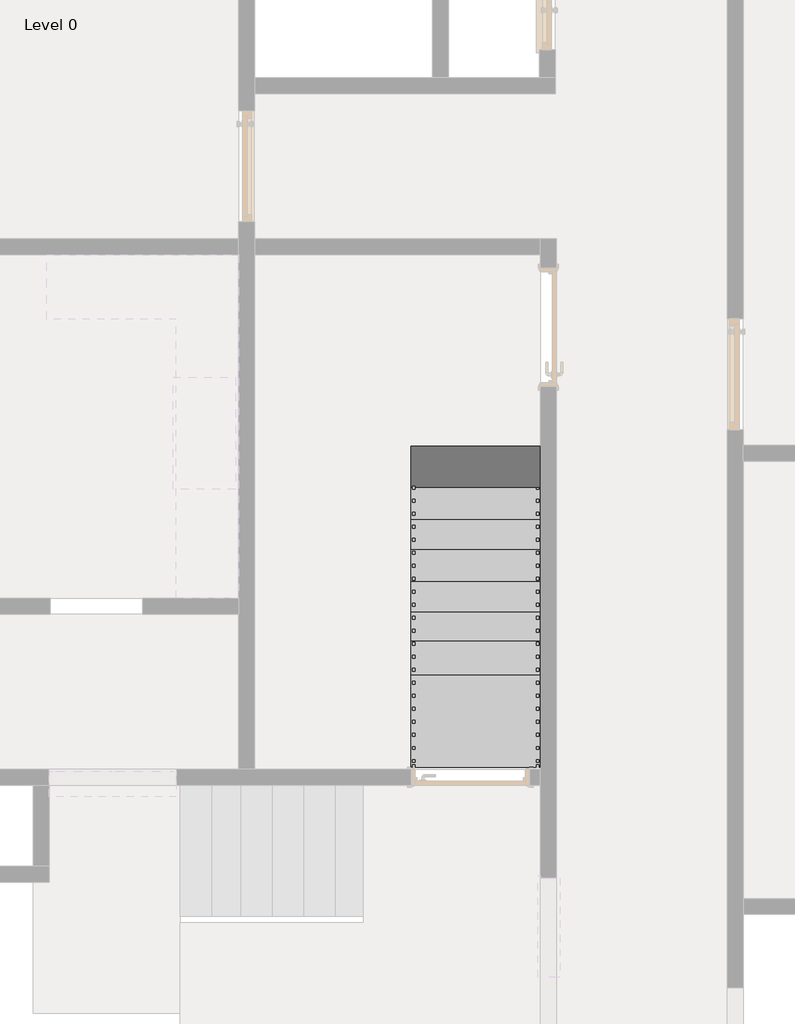
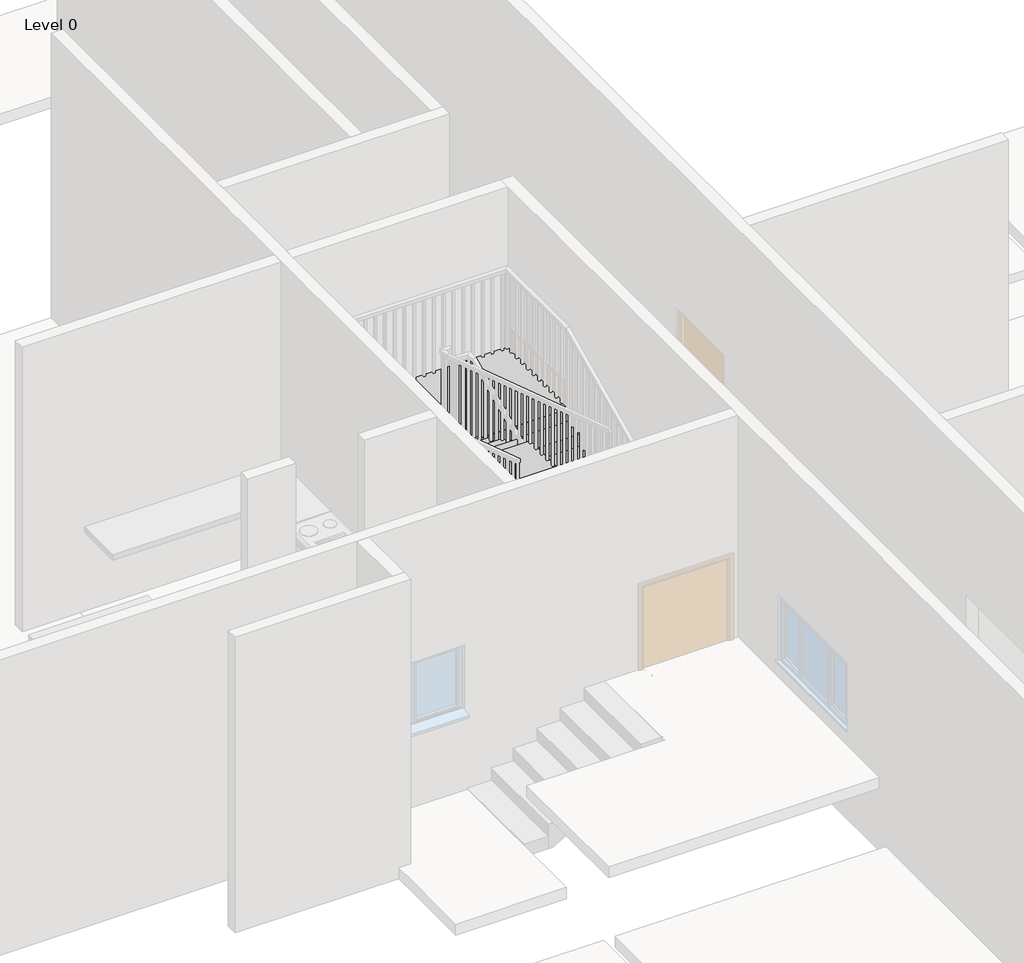
# One storey, part 10 of 14: 1 stair flight.
"""IFC4 building model written with IfcOpenShell, lengths in millimetres."""

from ifc_helpers import new_model, si_unit, frame, origin, place, context, project, spatial, polyline, outline, extrude, faceted_brep, element, save

model = new_model("IFC4")

# Units and contexts
model_context = context("Model", 3, world=origin())
ifc_project = project(units=[si_unit("LENGTHUNIT", "METRE", prefix="MILLI")], contexts=[model_context])

# Site, building, storey
site = spatial("IfcSite", under=ifc_project)
building = spatial("IfcBuilding", under=site)
storey = spatial("IfcBuildingStorey", under=building, Name="Level 0", Elevation=0.0)

# Stair flight
placement = place(None, origin())
element("IfcStairFlight", 1, ObjectType="1mm_Tread-175mm_Depth", at=placement, inside=storey, context=model_context, shape_type="SolidModel", body=[
    faceted_brep([(-22988.9547508, 26843.4116713, 165.6666667), (-22988.9547508, 25955.1270746, 165.6666667), (-21744.3547508, 25955.1270746, 165.6666667), (-21744.3547508, 26843.4116713, 165.6666667), (-22988.9547508, 26843.4116713, 0.0), (-22988.9547508, 25955.1270746, 0.0), (-21744.3547508, 25955.1270746, 0.0), (-21744.3547508, 26843.4116713, 0.0), (-22988.9547508, 26843.4116713, 332.3333333), (-21744.3547508, 26843.4116713, 332.3333333), (-21744.3547508, 26889.2374029, 332.3333333), (-21744.3547508, 27173.6116713, 332.3333333), (-22988.9547508, 27173.6116713, 332.3333333), (-22988.9547508, 26889.2374029, 332.3333333), (-22988.9547508, 27173.6116713, 150.5643087), (-22988.9547508, 26905.836521, 0.0), (-22988.9547508, 26889.2374029, 0.0), (-21744.3547508, 26889.2374029, 0.0), (-21744.3547508, 26905.836521, 0.0), (-21744.3547508, 27173.6116713, 150.5643087), (-22988.9547508, 27453.0116713, 499.0), (-22988.9547508, 27173.6116713, 499.0), (-21744.3547508, 27173.6116713, 499.0), (-21744.3547508, 27453.0116713, 499.0), (-22988.9547508, 27453.0116713, 307.6650247), (-21744.3547508, 27453.0116713, 307.6650247), (-22988.9547508, 27745.1116713, 665.6666667), (-22988.9547508, 27453.0116713, 665.6666667), (-21744.3547508, 27453.0116713, 665.6666667), (-21744.3547508, 27745.1116713, 665.6666667), (-22988.9547508, 27745.1116713, 471.9066824), (-21744.3547508, 27745.1116713, 471.9066824), (-22988.9547508, 28049.9116713, 832.3333333), (-22988.9547508, 27745.1116713, 832.3333333), (-21744.3547508, 27745.1116713, 832.3333333), (-21744.3547508, 28049.9116713, 832.3333333), (-22988.9547508, 28049.9116713, 643.2892817), (-21744.3547508, 28049.9116713, 643.2892817), (-22988.9547508, 28342.0116713, 999.0), (-22988.9547508, 28049.9116713, 999.0), (-21744.3547508, 28049.9116713, 999.0), (-21744.3547508, 28342.0116713, 999.0), (-22988.9547508, 28342.0116713, 807.5309394), (-21744.3547508, 28342.0116713, 807.5309394), (-22988.9547508, 28646.8116713, 1165.6666667), (-22988.9547508, 28342.0116713, 1165.6666667), (-21744.3547508, 28342.0116713, 1165.6666667), (-21744.3547508, 28646.8116713, 1165.6666667), (-22988.9547508, 28646.8116713, 978.9135387), (-21744.3547508, 28646.8116713, 978.9135387), (-22988.9547508, 28926.2116713, 1332.3333333), (-22988.9547508, 28646.8116713, 1332.3333333), (-21744.3547508, 28646.8116713, 1332.3333333), (-21744.3547508, 28926.2116713, 1332.3333333), (-22988.9547508, 28926.2116713, 1136.0142547), (-21744.3547508, 28926.2116713, 1136.0142547), (-22988.9547508, 29231.0116713, 1499.0), (-22988.9547508, 28926.2116713, 1499.0), (-21744.3547508, 28926.2116713, 1499.0), (-21744.3547508, 29231.0116713, 1499.0), (-22988.9547508, 29231.0116713, 1307.396854), (-21744.3547508, 29231.0116713, 1307.396854), (-22988.9547508, 29511.1270746, 1665.6666667), (-22988.9547508, 29231.0116713, 1665.6666667), (-21744.3547508, 29231.0116713, 1665.6666667), (-21744.3547508, 29511.1270746, 1665.6666667), (-22988.9547508, 29511.1270746, 1464.8998261), (-21744.3547508, 29511.1270746, 1464.8998261), (-23268.3547508, 29511.1270746, 1832.3333333), (-23268.3547508, 29612.7270746, 1832.3333333), (-22988.9547508, 29612.7270746, 1832.3333333), (-22988.9547508, 29511.1270746, 1832.3333333), (-21744.3547508, 29511.1270746, 1832.3333333), (-21744.3547508, 29853.3656288, 1832.3333333), (-21744.3547508, 30884.0294818, 1832.3333333), (-24494.5800447, 30884.0294818, 1832.3333333), (-24494.5800447, 29511.1270746, 1832.3333333), (-23268.3547508, 29511.1270746, 1657.3333333), (-23268.3547508, 29612.7270746, 1657.3333333), (-22988.9547508, 29612.7270746, 1657.3333333), (-22988.9547508, 29853.3656288, 1657.3333333), (-21744.3547508, 29853.3656288, 1657.3333333), (-21744.3547508, 30884.0294818, 1657.3333333), (-24494.5800447, 30884.0294818, 1657.3333333), (-24494.5800447, 29511.1270746, 1657.3333333), (-23268.3547508, 29511.1270746, 1999.0), (-24494.5800447, 29511.1270746, 1999.0), (-24494.5800447, 29465.0198504, 1999.0), (-24494.5800447, 29231.0116713, 1999.0), (-23268.3547508, 29231.0116713, 1999.0), (-23268.3547508, 29465.0198504, 1999.0), (-23268.3547508, 29231.0116713, 1789.8396403), (-23268.3547508, 29465.0198504, 1657.3333333), (-24494.5800447, 29465.0198504, 1657.3333333), (-24494.5800447, 29231.0116713, 1789.8396403), (-23268.3547508, 28926.2116713, 2165.6666667), (-23268.3547508, 29231.0116713, 2165.6666667), (-24494.5800447, 29231.0116713, 2165.6666667), (-24494.5800447, 28926.2116713, 2165.6666667), (-23268.3547508, 28926.2116713, 1962.4315664), (-24494.5800447, 28926.2116713, 1962.4315664), (-23268.3547508, 28646.8116713, 2332.3333333), (-23268.3547508, 28926.2116713, 2332.3333333), (-24494.5800447, 28926.2116713, 2332.3333333), (-24494.5800447, 28646.8116713, 2332.3333333), (-23268.3547508, 28646.8116713, 2120.640832), (-24494.5800447, 28646.8116713, 2120.640832), (-23268.3547508, 28342.0116713, 2499.0), (-23268.3547508, 28646.8116713, 2499.0), (-24494.5800447, 28646.8116713, 2499.0), (-24494.5800447, 28342.0116713, 2499.0), (-23268.3547508, 28342.0116713, 2293.2327581), (-24494.5800447, 28342.0116713, 2293.2327581), (-23268.3547508, 28049.9116713, 2665.6666667), (-23268.3547508, 28342.0116713, 2665.6666667), (-24494.5800447, 28342.0116713, 2665.6666667), (-24494.5800447, 28049.9116713, 2665.6666667), (-23268.3547508, 28049.9116713, 2458.6333539), (-24494.5800447, 28049.9116713, 2458.6333539), (-23268.3547508, 27745.1116713, 2832.3333333), (-23268.3547508, 28049.9116713, 2832.3333333), (-24494.5800447, 28049.9116713, 2832.3333333), (-24494.5800447, 27745.1116713, 2832.3333333), (-23268.3547508, 27745.1116713, 2631.2252801), (-24494.5800447, 27745.1116713, 2631.2252801), (-23268.3547508, 27745.1116713, 2999.0), (-24494.5800447, 27745.1116713, 2999.0), (-24494.5800447, 27404.6685466, 2999.0), (-24494.5800447, 25935.1270746, 2999.0), (-23268.3547508, 25935.1270746, 2999.0), (-23268.3547508, 27404.6685466, 2999.0), (-23268.3547508, 25935.1270746, 2824.0), (-23268.3547508, 27404.6685466, 2824.0), (-24494.5800447, 27404.6685466, 2824.0), (-24494.5800447, 25935.1270746, 2824.0)], [[[0, 1, 2, 3]], [[1, 0, 4, 5]], [[2, 1, 5, 6]], [[3, 2, 6, 7]], [[8, 9, 10, 11, 12, 13]], [[4, 0, 8, 13, 12, 14, 15, 16]], [[0, 3, 9, 8]], [[3, 7, 17, 18, 19, 11, 10, 9]], [[20, 21, 22, 23]], [[21, 20, 24, 14, 12]], [[12, 11, 22, 21]], [[23, 22, 11, 19, 25]], [[26, 27, 28, 29]], [[27, 26, 30, 24, 20]], [[20, 23, 28, 27]], [[29, 28, 23, 25, 31]], [[32, 33, 34, 35]], [[33, 32, 36, 30, 26]], [[26, 29, 34, 33]], [[35, 34, 29, 31, 37]], [[38, 39, 40, 41]], [[39, 38, 42, 36, 32]], [[32, 35, 40, 39]], [[41, 40, 35, 37, 43]], [[44, 45, 46, 47]], [[45, 44, 48, 42, 38]], [[38, 41, 46, 45]], [[47, 46, 41, 43, 49]], [[50, 51, 52, 53]], [[51, 50, 54, 48, 44]], [[44, 47, 52, 51]], [[53, 52, 47, 49, 55]], [[56, 57, 58, 59]], [[57, 56, 60, 54, 50]], [[50, 53, 58, 57]], [[59, 58, 53, 55, 61]], [[62, 63, 64, 65]], [[63, 62, 66, 60, 56]], [[56, 59, 64, 63]], [[65, 64, 59, 61, 67]], [[68, 69, 70, 71, 72, 73, 74, 75, 76]], [[69, 68, 77, 78]], [[70, 69, 78, 79]], [[71, 70, 79, 80, 66, 62]], [[62, 65, 72, 71]], [[72, 65, 67, 81, 82, 74, 73]], [[75, 74, 82, 83]], [[76, 75, 83, 84]], [[85, 86, 87, 88, 89, 90]], [[68, 85, 90, 89, 91, 92, 77]], [[68, 76, 86, 85]], [[86, 76, 84, 93, 94, 88, 87]], [[95, 96, 97, 98]], [[96, 95, 99, 91, 89]], [[89, 88, 97, 96]], [[98, 97, 88, 94, 100]], [[101, 102, 103, 104]], [[102, 101, 105, 99, 95]], [[95, 98, 103, 102]], [[104, 103, 98, 100, 106]], [[107, 108, 109, 110]], [[108, 107, 111, 105, 101]], [[101, 104, 109, 108]], [[110, 109, 104, 106, 112]], [[113, 114, 115, 116]], [[114, 113, 117, 111, 107]], [[107, 110, 115, 114]], [[116, 115, 110, 112, 118]], [[119, 120, 121, 122]], [[120, 119, 123, 117, 113]], [[113, 116, 121, 120]], [[122, 121, 116, 118, 124]], [[125, 126, 127, 128, 129, 130]], [[119, 125, 130, 129, 131, 132, 123]], [[119, 122, 126, 125]], [[126, 122, 124, 133, 134, 128, 127]], [[129, 128, 134, 131]], [[5, 4, 16, 15, 18, 17, 7, 6]], [[66, 80, 81, 67, 61, 55, 49, 43, 37, 31, 25, 19, 18, 15, 14, 24, 30, 36, 42, 48, 54, 60]], [[81, 80, 79, 78, 77, 92, 93, 84, 83, 82]], [[93, 92, 91, 99, 105, 111, 117, 123, 132, 133, 124, 118, 112, 106, 100, 94]], [[133, 132, 131, 134]]]),
    extrude(outline(polyline([(-22988.9547508, 26843.4116713), (-21744.3547508, 26843.4116713), (-21744.3547508, 25955.1270746), (-22988.9547508, 25955.1270746), (-22988.9547508, 26843.4116713)])), frame((0.0, 0.0, 165.6666667), z_axis=(0.0, 0.0, 1.0), x_axis=(1.0, 0.0, 0.0)), (0.0, 0.0, 1.0), 1.0),
    extrude(outline(polyline([(-22988.9547508, 27173.6116713), (-21744.3547508, 27173.6116713), (-21744.3547508, 26843.4116713), (-22988.9547508, 26843.4116713), (-22988.9547508, 27173.6116713)])), frame((0.0, 0.0, 332.3333333), z_axis=(0.0, 0.0, 1.0), x_axis=(1.0, 0.0, 0.0)), (0.0, 0.0, 1.0), 1.0),
    extrude(outline(polyline([(-22988.9547508, 27453.0116713), (-21744.3547508, 27453.0116713), (-21744.3547508, 27173.6116713), (-22988.9547508, 27173.6116713), (-22988.9547508, 27453.0116713)])), frame((0.0, 0.0, 499.0), z_axis=(0.0, 0.0, 1.0), x_axis=(1.0, 0.0, 0.0)), (0.0, 0.0, 1.0), 1.0),
    extrude(outline(polyline([(-22988.9547508, 27745.1116713), (-21744.3547508, 27745.1116713), (-21744.3547508, 27453.0116713), (-22988.9547508, 27453.0116713), (-22988.9547508, 27745.1116713)])), frame((0.0, 0.0, 665.6666667), z_axis=(0.0, 0.0, 1.0), x_axis=(1.0, 0.0, 0.0)), (0.0, 0.0, 1.0), 1.0),
    extrude(outline(polyline([(-22988.9547508, 28049.9116713), (-21744.3547508, 28049.9116713), (-21744.3547508, 27745.1116713), (-22988.9547508, 27745.1116713), (-22988.9547508, 28049.9116713)])), frame((0.0, 0.0, 832.3333333), z_axis=(0.0, 0.0, 1.0), x_axis=(1.0, 0.0, 0.0)), (0.0, 0.0, 1.0), 1.0),
    extrude(outline(polyline([(-22988.9547508, 28342.0116713), (-21744.3547508, 28342.0116713), (-21744.3547508, 28049.9116713), (-22988.9547508, 28049.9116713), (-22988.9547508, 28342.0116713)])), frame((0.0, 0.0, 999.0), z_axis=(0.0, 0.0, 1.0), x_axis=(1.0, 0.0, 0.0)), (0.0, 0.0, 1.0), 1.0),
    extrude(outline(polyline([(-22988.9547508, 28646.8116713), (-21744.3547508, 28646.8116713), (-21744.3547508, 28342.0116713), (-22988.9547508, 28342.0116713), (-22988.9547508, 28646.8116713)])), frame((0.0, 0.0, 1165.6666667), z_axis=(0.0, 0.0, 1.0), x_axis=(1.0, 0.0, 0.0)), (0.0, 0.0, 1.0), 1.0),
    extrude(outline(polyline([(-22988.9547508, 28926.2116713), (-21744.3547508, 28926.2116713), (-21744.3547508, 28646.8116713), (-22988.9547508, 28646.8116713), (-22988.9547508, 28926.2116713)])), frame((0.0, 0.0, 1332.3333333), z_axis=(0.0, 0.0, 1.0), x_axis=(1.0, 0.0, 0.0)), (0.0, 0.0, 1.0), 1.0),
    extrude(outline(polyline([(-22988.9547508, 29231.0116713), (-21744.3547508, 29231.0116713), (-21744.3547508, 28926.2116713), (-22988.9547508, 28926.2116713), (-22988.9547508, 29231.0116713)])), frame((0.0, 0.0, 1499.0), z_axis=(0.0, 0.0, 1.0), x_axis=(1.0, 0.0, 0.0)), (0.0, 0.0, 1.0), 1.0),
    extrude(outline(polyline([(-22988.9547508, 29511.1270746), (-21744.3547508, 29511.1270746), (-21744.3547508, 29231.0116713), (-22988.9547508, 29231.0116713), (-22988.9547508, 29511.1270746)])), frame((0.0, 0.0, 1665.6666667), z_axis=(0.0, 0.0, 1.0), x_axis=(1.0, 0.0, 0.0)), (0.0, 0.0, 1.0), 1.0),
    extrude(outline(polyline([(-23268.3547508, 29511.1270746), (-24494.5800447, 29511.1270746), (-24494.5800447, 30884.0294818), (-21744.3547508, 30884.0294818), (-21744.3547508, 29511.1270746), (-22988.9547508, 29511.1270746), (-22988.9547508, 29612.7270746), (-23268.3547508, 29612.7270746), (-23268.3547508, 29511.1270746)])), frame((0.0, 0.0, 1832.3333333), z_axis=(0.0, 0.0, 1.0), x_axis=(1.0, 0.0, 0.0)), (0.0, 0.0, 1.0), 1.0),
    extrude(outline(polyline([(-23268.3547508, 29231.0116713), (-24494.5800447, 29231.0116713), (-24494.5800447, 29511.1270746), (-23268.3547508, 29511.1270746), (-23268.3547508, 29231.0116713)])), frame((0.0, 0.0, 1999.0), z_axis=(0.0, 0.0, 1.0), x_axis=(1.0, 0.0, 0.0)), (0.0, 0.0, 1.0), 1.0),
    extrude(outline(polyline([(-23268.3547508, 28926.2116713), (-24494.5800447, 28926.2116713), (-24494.5800447, 29231.0116713), (-23268.3547508, 29231.0116713), (-23268.3547508, 28926.2116713)])), frame((0.0, 0.0, 2165.6666667), z_axis=(0.0, 0.0, 1.0), x_axis=(1.0, 0.0, 0.0)), (0.0, 0.0, 1.0), 1.0),
    extrude(outline(polyline([(-23268.3547508, 28646.8116713), (-24494.5800447, 28646.8116713), (-24494.5800447, 28926.2116713), (-23268.3547508, 28926.2116713), (-23268.3547508, 28646.8116713)])), frame((0.0, 0.0, 2332.3333333), z_axis=(0.0, 0.0, 1.0), x_axis=(1.0, 0.0, 0.0)), (0.0, 0.0, 1.0), 1.0),
    extrude(outline(polyline([(-23268.3547508, 28342.0116713), (-24494.5800447, 28342.0116713), (-24494.5800447, 28646.8116713), (-23268.3547508, 28646.8116713), (-23268.3547508, 28342.0116713)])), frame((0.0, 0.0, 2499.0), z_axis=(0.0, 0.0, 1.0), x_axis=(1.0, 0.0, 0.0)), (0.0, 0.0, 1.0), 1.0),
    extrude(outline(polyline([(-23268.3547508, 28049.9116713), (-24494.5800447, 28049.9116713), (-24494.5800447, 28342.0116713), (-23268.3547508, 28342.0116713), (-23268.3547508, 28049.9116713)])), frame((0.0, 0.0, 2665.6666667), z_axis=(0.0, 0.0, 1.0), x_axis=(1.0, 0.0, 0.0)), (0.0, 0.0, 1.0), 1.0),
    extrude(outline(polyline([(-23268.3547508, 27745.1116713), (-24494.5800447, 27745.1116713), (-24494.5800447, 28049.9116713), (-23268.3547508, 28049.9116713), (-23268.3547508, 27745.1116713)])), frame((0.0, 0.0, 2832.3333333), z_axis=(0.0, 0.0, 1.0), x_axis=(1.0, 0.0, 0.0)), (0.0, 0.0, 1.0), 1.0),
    extrude(outline(polyline([(-23268.3547508, 25935.1270746), (-24494.5800447, 25935.1270746), (-24494.5800447, 27745.1116713), (-23268.3547508, 27745.1116713), (-23268.3547508, 25935.1270746)])), frame((0.0, 0.0, 2999.0), z_axis=(0.0, 0.0, 1.0), x_axis=(1.0, 0.0, 0.0)), (0.0, 0.0, 1.0), 1.0),
])

save(model, "model.ifc")

# Revit data of these elements
# Element 1 (IfcStairFlight, "1mm_Tread-175mm_Depth")
#   Phase Created = New Construction
#   Materials on its faces: "Concrete, Cast-in-Place gray"
# Materials
#   "Concrete, Cast-in-Place gray": class "Concrete", colour RGB 192 192 192, transparency 0, Description = "Cast-in-place concrete", Cost = 0
